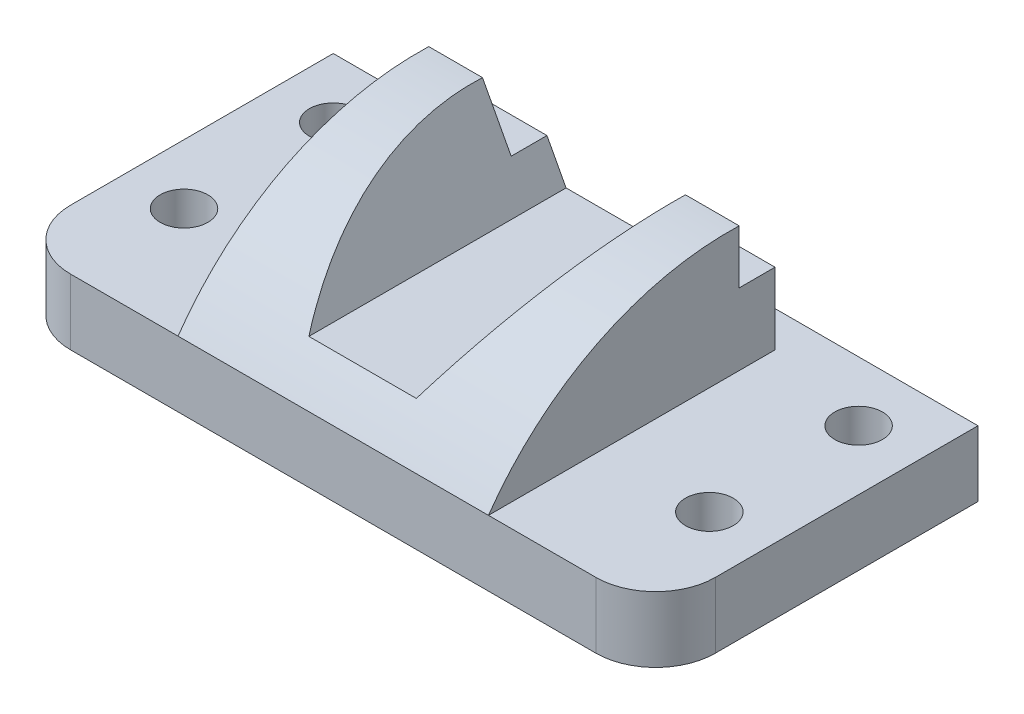
ISO-10303-21;
HEADER;
FILE_DESCRIPTION(('STEP AP214'),'2;1');
FILE_NAME('part.step','',(''),(''),'','','');
FILE_SCHEMA(('AUTOMOTIVE_DESIGN { 1 0 10303 214 1 1 1 1 }'));
ENDSEC;
DATA;
#1=APPLICATION_CONTEXT('core data for automotive mechanical design processes');
#2=APPLICATION_PROTOCOL_DEFINITION('international standard','automotive_design',2000,#1);
#3=PRODUCT_CONTEXT('',#1,'mechanical');
#4=PRODUCT('Part','Part','',(#3));
#5=PRODUCT_RELATED_PRODUCT_CATEGORY('part','',(#4));
#6=PRODUCT_DEFINITION_FORMATION('','',#4);
#7=PRODUCT_DEFINITION_CONTEXT('part definition',#1,'design');
#8=PRODUCT_DEFINITION('design','',#6,#7);
#9=PRODUCT_DEFINITION_SHAPE('','',#8);
#10=(LENGTH_UNIT() NAMED_UNIT(*) SI_UNIT(.MILLI.,.METRE.));
#11=(NAMED_UNIT(*) PLANE_ANGLE_UNIT() SI_UNIT($,.RADIAN.));
#12=(NAMED_UNIT(*) SI_UNIT($,.STERADIAN.) SOLID_ANGLE_UNIT());
#13=UNCERTAINTY_MEASURE_WITH_UNIT(LENGTH_MEASURE(1.E-05),#10,'distance_accuracy_value','');
#14=(GEOMETRIC_REPRESENTATION_CONTEXT(3) GLOBAL_UNCERTAINTY_ASSIGNED_CONTEXT((#13)) GLOBAL_UNIT_ASSIGNED_CONTEXT((#10,
#11,#12)) REPRESENTATION_CONTEXT('',''));
#15=CARTESIAN_POINT('',(0.,0.,0.));
#16=DIRECTION('',(0.,0.,1.));
#17=DIRECTION('',(1.,0.,0.));
#18=AXIS2_PLACEMENT_3D('',#15,#16,#17);
#19=CARTESIAN_POINT('',(-26.,72.,-21.));
#20=DIRECTION('',(0.,0.,1.));
#21=DIRECTION('',(1.,0.,0.));
#22=AXIS2_PLACEMENT_3D('',#19,#20,#21);
#23=PLANE('',#22);
#24=DIRECTION('',(-0.470588235294119,0.88235294117647,0.));
#25=VECTOR('',#24,1.);
#26=CARTESIAN_POINT('',(-35.6020761245675,66.878892733564,-21.));
#27=LINE('',#26,#25);
#28=CARTESIAN_POINT('',(-9.,17.,-21.));
#29=VERTEX_POINT('',#28);
#30=CARTESIAN_POINT('',(-12.2,23.,-21.));
#31=VERTEX_POINT('',#30);
#32=EDGE_CURVE('E178',#29,#31,#27,.T.);
#33=ORIENTED_EDGE('',*,*,#32,.F.);
#34=DIRECTION('',(1.,0.,0.));
#35=VECTOR('',#34,1.);
#36=CARTESIAN_POINT('',(-26.,17.,-21.));
#37=LINE('',#36,#35);
#38=CARTESIAN_POINT('',(9.,17.,-21.));
#39=VERTEX_POINT('',#38);
#40=EDGE_CURVE('E166',#29,#39,#37,.T.);
#41=ORIENTED_EDGE('',*,*,#40,.T.);
#42=DIRECTION('',(0.470588235294118,0.88235294117647,0.));
#43=VECTOR('',#42,1.);
#44=CARTESIAN_POINT('',(24.0865051903114,45.2871972318339,-21.));
#45=LINE('',#44,#43);
#46=CARTESIAN_POINT('',(12.2,23.,-21.));
#47=VERTEX_POINT('',#46);
#48=EDGE_CURVE('E152',#39,#47,#45,.T.);
#49=ORIENTED_EDGE('',*,*,#48,.T.);
#50=DIRECTION('',(1.,0.,0.));
#51=VECTOR('',#50,1.);
#52=CARTESIAN_POINT('',(-35.,23.,-21.));
#53=LINE('',#52,#51);
#54=CARTESIAN_POINT('',(26.,23.,-21.));
#55=VERTEX_POINT('',#54);
#56=EDGE_CURVE('E191',#47,#55,#53,.T.);
#57=ORIENTED_EDGE('',*,*,#56,.T.);
#58=DIRECTION('',(0.,-1.,0.));
#59=VECTOR('',#58,1.);
#60=CARTESIAN_POINT('',(26.,72.,-21.));
#61=LINE('',#60,#59);
#62=CARTESIAN_POINT('',(26.,11.,-21.));
#63=VERTEX_POINT('',#62);
#64=EDGE_CURVE('E211',#55,#63,#61,.T.);
#65=ORIENTED_EDGE('',*,*,#64,.T.);
#66=DIRECTION('',(-1.,0.,0.));
#67=VECTOR('',#66,1.);
#68=CARTESIAN_POINT('',(-26.,11.,-21.));
#69=LINE('',#68,#67);
#70=CARTESIAN_POINT('',(-26.,11.,-21.));
#71=VERTEX_POINT('',#70);
#72=EDGE_CURVE('E202',#63,#71,#69,.T.);
#73=ORIENTED_EDGE('',*,*,#72,.T.);
#74=DIRECTION('',(0.,-1.,0.));
#75=VECTOR('',#74,1.);
#76=CARTESIAN_POINT('',(-26.,72.,-21.));
#77=LINE('',#76,#75);
#78=CARTESIAN_POINT('',(-26.,23.,-21.));
#79=VERTEX_POINT('',#78);
#80=EDGE_CURVE('E65',#79,#71,#77,.T.);
#81=ORIENTED_EDGE('',*,*,#80,.F.);
#82=EDGE_CURVE('E194',#79,#31,#53,.T.);
#83=ORIENTED_EDGE('',*,*,#82,.T.);
#84=EDGE_LOOP('',(#33,#41,#49,#57,#65,#73,#81,#83));
#85=FACE_BOUND('',#84,.T.);
#86=ADVANCED_FACE('F39',(#85),#23,.F.);
#87=CARTESIAN_POINT('',(-35.,23.,-21.));
#88=DIRECTION('',(0.,-1.,0.));
#89=DIRECTION('',(0.,0.,-1.));
#90=AXIS2_PLACEMENT_3D('',#87,#88,#89);
#91=PLANE('',#90);
#92=DIRECTION('',(0.,0.,1.));
#93=VECTOR('',#92,1.);
#94=CARTESIAN_POINT('',(-12.2,23.,-21.));
#95=LINE('',#94,#93);
#96=CARTESIAN_POINT('',(-12.2,23.,-15.));
#97=VERTEX_POINT('',#96);
#98=EDGE_CURVE('E185',#31,#97,#95,.T.);
#99=ORIENTED_EDGE('',*,*,#98,.F.);
#100=ORIENTED_EDGE('',*,*,#82,.F.);
#101=DIRECTION('',(0.,0.,-1.));
#102=VECTOR('',#101,1.);
#103=CARTESIAN_POINT('',(-26.,23.,27.));
#104=LINE('',#103,#102);
#105=CARTESIAN_POINT('',(-26.,23.,-15.));
#106=VERTEX_POINT('',#105);
#107=EDGE_CURVE('E287',#106,#79,#104,.T.);
#108=ORIENTED_EDGE('',*,*,#107,.F.);
#109=DIRECTION('',(1.,0.,0.));
#110=VECTOR('',#109,1.);
#111=CARTESIAN_POINT('',(-35.,23.,-15.));
#112=LINE('',#111,#110);
#113=EDGE_CURVE('E198',#106,#97,#112,.T.);
#114=ORIENTED_EDGE('',*,*,#113,.T.);
#115=EDGE_LOOP('',(#99,#100,#108,#114));
#116=FACE_BOUND('',#115,.T.);
#117=ADVANCED_FACE('F313',(#116),#91,.F.);
#118=CARTESIAN_POINT('',(-35.,23.,-15.));
#119=DIRECTION('',(0.,0.,1.));
#120=DIRECTION('',(1.,0.,0.));
#121=AXIS2_PLACEMENT_3D('',#118,#119,#120);
#122=PLANE('',#121);
#123=DIRECTION('',(-0.470588235294119,0.88235294117647,0.));
#124=VECTOR('',#123,1.);
#125=CARTESIAN_POINT('',(-17.2491349480969,32.4671280276817,-15.));
#126=LINE('',#125,#124);
#127=CARTESIAN_POINT('',(-17.,32.,-15.));
#128=VERTEX_POINT('',#127);
#129=EDGE_CURVE('E162',#97,#128,#126,.T.);
#130=ORIENTED_EDGE('',*,*,#129,.F.);
#131=ORIENTED_EDGE('',*,*,#113,.F.);
#132=DIRECTION('',(0.,-1.,0.));
#133=VECTOR('',#132,1.);
#134=CARTESIAN_POINT('',(-26.,72.,-15.));
#135=LINE('',#134,#133);
#136=CARTESIAN_POINT('',(-26.,32.,-15.));
#137=VERTEX_POINT('',#136);
#138=EDGE_CURVE('E284',#137,#106,#135,.T.);
#139=ORIENTED_EDGE('',*,*,#138,.F.);
#140=DIRECTION('',(1.,0.,0.));
#141=VECTOR('',#140,1.);
#142=CARTESIAN_POINT('',(-35.,32.,-15.));
#143=LINE('',#142,#141);
#144=EDGE_CURVE('E53',#137,#128,#143,.T.);
#145=ORIENTED_EDGE('',*,*,#144,.T.);
#146=EDGE_LOOP('',(#130,#131,#139,#145));
#147=FACE_BOUND('',#146,.T.);
#148=ADVANCED_FACE('F309',(#147),#122,.F.);
#149=CARTESIAN_POINT('',(-35.,-16.9681686592954,-13.2340843296477));
#150=DIRECTION('',(1.,0.,0.));
#151=DIRECTION('',(0.,0.,-1.));
#152=AXIS2_PLACEMENT_3D('',#149,#150,#151);
#153=CYLINDRICAL_SURFACE('',#152,49.);
#154=CARTESIAN_POINT('',(9.11635661829097,-16.9681686592954,-13.2340843296477));
#155=DIRECTION('',(0.88235294117647,0.470588235294119,0.));
#156=DIRECTION('',(0.470588235294119,-0.88235294117647,0.));
#157=AXIS2_PLACEMENT_3D('',#154,#155,#156);
#158=ELLIPSE('',#157,55.5333333333334,49.);
#159=CARTESIAN_POINT('',(-9.,17.,22.0811180332676));
#160=VERTEX_POINT('',#159);
#161=EDGE_CURVE('E11',#128,#160,#158,.T.);
#162=ORIENTED_EDGE('',*,*,#161,.F.);
#163=ORIENTED_EDGE('',*,*,#144,.F.);
#164=CARTESIAN_POINT('',(-26.,-16.9681686592954,-13.2340843296477));
#165=DIRECTION('',(1.,0.,0.));
#166=DIRECTION('',(0.,0.,-1.));
#167=AXIS2_PLACEMENT_3D('',#164,#165,#166);
#168=CIRCLE('',#167,49.);
#169=CARTESIAN_POINT('',(-26.,11.,27.));
#170=VERTEX_POINT('',#169);
#171=EDGE_CURVE('E285',#170,#137,#168,.F.);
#172=ORIENTED_EDGE('',*,*,#171,.F.);
#173=DIRECTION('',(1.,0.,0.));
#174=VECTOR('',#173,1.);
#175=CARTESIAN_POINT('',(-35.,11.,27.));
#176=LINE('',#175,#174);
#177=CARTESIAN_POINT('',(26.,11.,27.));
#178=VERTEX_POINT('',#177);
#179=EDGE_CURVE('E193',#170,#178,#176,.T.);
#180=ORIENTED_EDGE('',*,*,#179,.T.);
#181=CARTESIAN_POINT('',(26.,-16.9681686592954,-13.2340843296477));
#182=DIRECTION('',(-1.,0.,0.));
#183=DIRECTION('',(0.,0.,-1.));
#184=AXIS2_PLACEMENT_3D('',#181,#182,#183);
#185=CIRCLE('',#184,49.);
#186=CARTESIAN_POINT('',(26.,32.,-15.));
#187=VERTEX_POINT('',#186);
#188=EDGE_CURVE('E179',#178,#187,#185,.T.);
#189=ORIENTED_EDGE('',*,*,#188,.T.);
#190=CARTESIAN_POINT('',(17.,32.,-15.));
#191=VERTEX_POINT('',#190);
#192=EDGE_CURVE('E203',#191,#187,#143,.T.);
#193=ORIENTED_EDGE('',*,*,#192,.F.);
#194=CARTESIAN_POINT('',(-9.11635661829093,-16.9681686592954,-13.2340843296477));
#195=DIRECTION('',(0.88235294117647,-0.470588235294118,0.));
#196=DIRECTION('',(0.470588235294118,0.88235294117647,0.));
#197=AXIS2_PLACEMENT_3D('',#194,#195,#196);
#198=ELLIPSE('',#197,55.5333333333334,49.);
#199=CARTESIAN_POINT('',(9.,17.,22.0811180332676));
#200=VERTEX_POINT('',#199);
#201=EDGE_CURVE('E286',#191,#200,#198,.T.);
#202=ORIENTED_EDGE('',*,*,#201,.T.);
#203=DIRECTION('',(1.,0.,0.));
#204=VECTOR('',#203,1.);
#205=CARTESIAN_POINT('',(-35.,17.,22.0811180332676));
#206=LINE('',#205,#204);
#207=EDGE_CURVE('E50',#200,#160,#206,.F.);
#208=ORIENTED_EDGE('',*,*,#207,.T.);
#209=EDGE_LOOP('',(#162,#163,#172,#180,#189,#193,#202,#208));
#210=FACE_BOUND('',#209,.T.);
#211=ADVANCED_FACE('F292',(#210),#153,.T.);
#212=CARTESIAN_POINT('',(26.,72.,-21.));
#213=DIRECTION('',(-1.,0.,0.));
#214=DIRECTION('',(0.,0.,1.));
#215=AXIS2_PLACEMENT_3D('',#212,#213,#214);
#216=PLANE('',#215);
#217=ORIENTED_EDGE('',*,*,#64,.F.);
#218=DIRECTION('',(0.,0.,-1.));
#219=VECTOR('',#218,1.);
#220=CARTESIAN_POINT('',(26.,23.,-21.));
#221=LINE('',#220,#219);
#222=CARTESIAN_POINT('',(26.,23.,-15.));
#223=VERTEX_POINT('',#222);
#224=EDGE_CURVE('E186',#223,#55,#221,.T.);
#225=ORIENTED_EDGE('',*,*,#224,.F.);
#226=DIRECTION('',(0.,-1.,0.));
#227=VECTOR('',#226,1.);
#228=CARTESIAN_POINT('',(26.,23.,-15.));
#229=LINE('',#228,#227);
#230=EDGE_CURVE('E176',#187,#223,#229,.T.);
#231=ORIENTED_EDGE('',*,*,#230,.F.);
#232=ORIENTED_EDGE('',*,*,#188,.F.);
#233=DIRECTION('',(0.,0.,-1.));
#234=VECTOR('',#233,1.);
#235=CARTESIAN_POINT('',(26.,11.,-21.));
#236=LINE('',#235,#234);
#237=EDGE_CURVE('E195',#178,#63,#236,.T.);
#238=ORIENTED_EDGE('',*,*,#237,.T.);
#239=EDGE_LOOP('',(#217,#225,#231,#232,#238));
#240=FACE_BOUND('',#239,.T.);
#241=ADVANCED_FACE('F321',(#240),#216,.F.);
#242=CARTESIAN_POINT('',(-26.,72.,27.));
#243=DIRECTION('',(1.,0.,0.));
#244=DIRECTION('',(0.,0.,-1.));
#245=AXIS2_PLACEMENT_3D('',#242,#243,#244);
#246=PLANE('',#245);
#247=ORIENTED_EDGE('',*,*,#138,.T.);
#248=ORIENTED_EDGE('',*,*,#107,.T.);
#249=ORIENTED_EDGE('',*,*,#80,.T.);
#250=DIRECTION('',(0.,0.,1.));
#251=VECTOR('',#250,1.);
#252=CARTESIAN_POINT('',(-26.,11.,27.));
#253=LINE('',#252,#251);
#254=EDGE_CURVE('E208',#71,#170,#253,.T.);
#255=ORIENTED_EDGE('',*,*,#254,.T.);
#256=ORIENTED_EDGE('',*,*,#171,.T.);
#257=EDGE_LOOP('',(#247,#248,#249,#255,#256));
#258=FACE_BOUND('',#257,.T.);
#259=ADVANCED_FACE('F315',(#258),#246,.F.);
#260=CARTESIAN_POINT('',(-44.,11.,17.));
#261=DIRECTION('',(0.,-1.,0.));
#262=DIRECTION('',(0.,0.,-1.));
#263=AXIS2_PLACEMENT_3D('',#260,#261,#262);
#264=PLANE('',#263);
#265=CARTESIAN_POINT('',(44.,11.,8.00000000000001));
#266=DIRECTION('',(0.,1.,0.));
#267=DIRECTION('',(0.,0.,1.));
#268=AXIS2_PLACEMENT_3D('',#265,#266,#267);
#269=CIRCLE('',#268,4.00000000000001);
#270=CARTESIAN_POINT('',(44.,11.,12.));
#271=VERTEX_POINT('',#270);
#272=EDGE_CURVE('E212',#271,#271,#269,.T.);
#273=ORIENTED_EDGE('',*,*,#272,.F.);
#274=EDGE_LOOP('',(#273));
#275=FACE_BOUND('',#274,.T.);
#276=CARTESIAN_POINT('',(44.,11.,-17.));
#277=DIRECTION('',(0.,1.,0.));
#278=DIRECTION('',(0.,0.,1.));
#279=AXIS2_PLACEMENT_3D('',#276,#277,#278);
#280=CIRCLE('',#279,4.00000000000001);
#281=CARTESIAN_POINT('',(44.,11.,-13.));
#282=VERTEX_POINT('',#281);
#283=EDGE_CURVE('E219',#282,#282,#280,.T.);
#284=ORIENTED_EDGE('',*,*,#283,.F.);
#285=EDGE_LOOP('',(#284));
#286=FACE_BOUND('',#285,.T.);
#287=CARTESIAN_POINT('',(-44.,11.,8.00000000000001));
#288=DIRECTION('',(0.,1.,0.));
#289=DIRECTION('',(0.,0.,1.));
#290=AXIS2_PLACEMENT_3D('',#287,#288,#289);
#291=CIRCLE('',#290,4.00000000000001);
#292=CARTESIAN_POINT('',(-44.,11.,12.));
#293=VERTEX_POINT('',#292);
#294=EDGE_CURVE('E228',#293,#293,#291,.T.);
#295=ORIENTED_EDGE('',*,*,#294,.F.);
#296=EDGE_LOOP('',(#295));
#297=FACE_BOUND('',#296,.T.);
#298=CARTESIAN_POINT('',(-44.,11.,-17.));
#299=DIRECTION('',(0.,1.,0.));
#300=DIRECTION('',(0.,0.,1.));
#301=AXIS2_PLACEMENT_3D('',#298,#299,#300);
#302=CIRCLE('',#301,4.00000000000001);
#303=CARTESIAN_POINT('',(-44.,11.,-13.));
#304=VERTEX_POINT('',#303);
#305=EDGE_CURVE('E234',#304,#304,#302,.T.);
#306=ORIENTED_EDGE('',*,*,#305,.F.);
#307=EDGE_LOOP('',(#306));
#308=FACE_BOUND('',#307,.T.);
#309=ORIENTED_EDGE('',*,*,#254,.F.);
#310=ORIENTED_EDGE('',*,*,#72,.F.);
#311=ORIENTED_EDGE('',*,*,#237,.F.);
#312=DIRECTION('',(1.,0.,0.));
#313=VECTOR('',#312,1.);
#314=CARTESIAN_POINT('',(-43.9999999999999,11.,27.));
#315=LINE('',#314,#313);
#316=CARTESIAN_POINT('',(43.9999999999999,11.,27.));
#317=VERTEX_POINT('',#316);
#318=EDGE_CURVE('E247',#178,#317,#315,.T.);
#319=ORIENTED_EDGE('',*,*,#318,.T.);
#320=CARTESIAN_POINT('',(44.,11.,17.));
#321=DIRECTION('',(0.,1.,0.));
#322=DIRECTION('',(0.,0.,1.));
#323=AXIS2_PLACEMENT_3D('',#320,#321,#322);
#324=CIRCLE('',#323,10.);
#325=CARTESIAN_POINT('',(54.,11.,16.9999999999999));
#326=VERTEX_POINT('',#325);
#327=EDGE_CURVE('E253',#317,#326,#324,.T.);
#328=ORIENTED_EDGE('',*,*,#327,.T.);
#329=DIRECTION('',(0.,0.,-1.));
#330=VECTOR('',#329,1.);
#331=CARTESIAN_POINT('',(54.,11.,16.9999999999999));
#332=LINE('',#331,#330);
#333=CARTESIAN_POINT('',(54.,11.,-27.));
#334=VERTEX_POINT('',#333);
#335=EDGE_CURVE('E236',#326,#334,#332,.T.);
#336=ORIENTED_EDGE('',*,*,#335,.T.);
#337=DIRECTION('',(-1.,0.,0.));
#338=VECTOR('',#337,1.);
#339=CARTESIAN_POINT('',(-54.,11.,-27.));
#340=LINE('',#339,#338);
#341=CARTESIAN_POINT('',(-54.,11.,-27.));
#342=VERTEX_POINT('',#341);
#343=EDGE_CURVE('E243',#334,#342,#340,.T.);
#344=ORIENTED_EDGE('',*,*,#343,.T.);
#345=DIRECTION('',(0.,0.,1.));
#346=VECTOR('',#345,1.);
#347=CARTESIAN_POINT('',(-54.,11.,16.9999999999999));
#348=LINE('',#347,#346);
#349=CARTESIAN_POINT('',(-54.,11.,16.9999999999999));
#350=VERTEX_POINT('',#349);
#351=EDGE_CURVE('E242',#342,#350,#348,.T.);
#352=ORIENTED_EDGE('',*,*,#351,.T.);
#353=CARTESIAN_POINT('',(-44.,11.,17.));
#354=DIRECTION('',(0.,1.,0.));
#355=DIRECTION('',(0.,0.,-1.));
#356=AXIS2_PLACEMENT_3D('',#353,#354,#355);
#357=CIRCLE('',#356,10.);
#358=CARTESIAN_POINT('',(-43.9999999999999,11.,27.));
#359=VERTEX_POINT('',#358);
#360=EDGE_CURVE('E248',#350,#359,#357,.T.);
#361=ORIENTED_EDGE('',*,*,#360,.T.);
#362=EDGE_CURVE('E250',#359,#170,#315,.T.);
#363=ORIENTED_EDGE('',*,*,#362,.T.);
#364=EDGE_LOOP('',(#309,#310,#311,#319,#328,#336,#344,#352,#361,#363));
#365=FACE_BOUND('',#364,.T.);
#366=ADVANCED_FACE('F320',(#275,#286,#297,#308,#365),#264,.F.);
#367=CARTESIAN_POINT('',(-44.,0.,17.));
#368=DIRECTION('',(0.,-1.,0.));
#369=DIRECTION('',(0.,0.,-1.));
#370=AXIS2_PLACEMENT_3D('',#367,#368,#369);
#371=PLANE('',#370);
#372=CARTESIAN_POINT('',(44.,0.,-17.));
#373=DIRECTION('',(0.,1.,0.));
#374=DIRECTION('',(0.,0.,1.));
#375=AXIS2_PLACEMENT_3D('',#372,#373,#374);
#376=CIRCLE('',#375,4.00000000000001);
#377=CARTESIAN_POINT('',(44.,0.,-13.));
#378=VERTEX_POINT('',#377);
#379=EDGE_CURVE('E220',#378,#378,#376,.T.);
#380=ORIENTED_EDGE('',*,*,#379,.T.);
#381=EDGE_LOOP('',(#380));
#382=FACE_BOUND('',#381,.T.);
#383=CARTESIAN_POINT('',(-44.,0.,-17.));
#384=DIRECTION('',(0.,1.,0.));
#385=DIRECTION('',(0.,0.,1.));
#386=AXIS2_PLACEMENT_3D('',#383,#384,#385);
#387=CIRCLE('',#386,4.00000000000001);
#388=CARTESIAN_POINT('',(-44.,0.,-13.));
#389=VERTEX_POINT('',#388);
#390=EDGE_CURVE('E227',#389,#389,#387,.T.);
#391=ORIENTED_EDGE('',*,*,#390,.T.);
#392=EDGE_LOOP('',(#391));
#393=FACE_BOUND('',#392,.T.);
#394=DIRECTION('',(0.,0.,-1.));
#395=VECTOR('',#394,1.);
#396=CARTESIAN_POINT('',(54.,0.,16.9999999999999));
#397=LINE('',#396,#395);
#398=CARTESIAN_POINT('',(54.,0.,16.9999999999999));
#399=VERTEX_POINT('',#398);
#400=CARTESIAN_POINT('',(54.,0.,-27.));
#401=VERTEX_POINT('',#400);
#402=EDGE_CURVE('E231',#399,#401,#397,.T.);
#403=ORIENTED_EDGE('',*,*,#402,.F.);
#404=CARTESIAN_POINT('',(44.,0.,17.));
#405=DIRECTION('',(0.,1.,0.));
#406=DIRECTION('',(0.,0.,1.));
#407=AXIS2_PLACEMENT_3D('',#404,#405,#406);
#408=CIRCLE('',#407,10.);
#409=CARTESIAN_POINT('',(43.9999999999999,0.,27.));
#410=VERTEX_POINT('',#409);
#411=EDGE_CURVE('E245',#410,#399,#408,.T.);
#412=ORIENTED_EDGE('',*,*,#411,.F.);
#413=DIRECTION('',(1.,0.,0.));
#414=VECTOR('',#413,1.);
#415=CARTESIAN_POINT('',(-43.9999999999999,0.,27.));
#416=LINE('',#415,#414);
#417=CARTESIAN_POINT('',(-43.9999999999999,0.,27.));
#418=VERTEX_POINT('',#417);
#419=EDGE_CURVE('E265',#418,#410,#416,.T.);
#420=ORIENTED_EDGE('',*,*,#419,.F.);
#421=CARTESIAN_POINT('',(-44.,0.,17.));
#422=DIRECTION('',(0.,1.,0.));
#423=DIRECTION('',(0.,0.,-1.));
#424=AXIS2_PLACEMENT_3D('',#421,#422,#423);
#425=CIRCLE('',#424,10.);
#426=CARTESIAN_POINT('',(-54.,0.,16.9999999999999));
#427=VERTEX_POINT('',#426);
#428=EDGE_CURVE('E257',#427,#418,#425,.T.);
#429=ORIENTED_EDGE('',*,*,#428,.F.);
#430=DIRECTION('',(0.,0.,1.));
#431=VECTOR('',#430,1.);
#432=CARTESIAN_POINT('',(-54.,0.,16.9999999999999));
#433=LINE('',#432,#431);
#434=CARTESIAN_POINT('',(-54.,0.,-27.));
#435=VERTEX_POINT('',#434);
#436=EDGE_CURVE('E256',#435,#427,#433,.T.);
#437=ORIENTED_EDGE('',*,*,#436,.F.);
#438=DIRECTION('',(-1.,0.,0.));
#439=VECTOR('',#438,1.);
#440=CARTESIAN_POINT('',(-54.,0.,-27.));
#441=LINE('',#440,#439);
#442=EDGE_CURVE('E258',#401,#435,#441,.T.);
#443=ORIENTED_EDGE('',*,*,#442,.F.);
#444=EDGE_LOOP('',(#403,#412,#420,#429,#437,#443));
#445=FACE_BOUND('',#444,.T.);
#446=CARTESIAN_POINT('',(-44.,0.,8.00000000000001));
#447=DIRECTION('',(0.,1.,0.));
#448=DIRECTION('',(0.,0.,1.));
#449=AXIS2_PLACEMENT_3D('',#446,#447,#448);
#450=CIRCLE('',#449,4.00000000000001);
#451=CARTESIAN_POINT('',(-44.,0.,12.));
#452=VERTEX_POINT('',#451);
#453=EDGE_CURVE('E224',#452,#452,#450,.T.);
#454=ORIENTED_EDGE('',*,*,#453,.T.);
#455=EDGE_LOOP('',(#454));
#456=FACE_BOUND('',#455,.T.);
#457=CARTESIAN_POINT('',(44.,0.,8.00000000000001));
#458=DIRECTION('',(0.,1.,0.));
#459=DIRECTION('',(0.,0.,1.));
#460=AXIS2_PLACEMENT_3D('',#457,#458,#459);
#461=CIRCLE('',#460,4.00000000000001);
#462=CARTESIAN_POINT('',(44.,0.,12.));
#463=VERTEX_POINT('',#462);
#464=EDGE_CURVE('E213',#463,#463,#461,.T.);
#465=ORIENTED_EDGE('',*,*,#464,.T.);
#466=EDGE_LOOP('',(#465));
#467=FACE_BOUND('',#466,.T.);
#468=ADVANCED_FACE('F351',(#382,#393,#445,#456,#467),#371,.T.);
#469=CARTESIAN_POINT('',(54.,11.,16.9999999999999));
#470=DIRECTION('',(-1.,0.,0.));
#471=DIRECTION('',(0.,0.,1.));
#472=AXIS2_PLACEMENT_3D('',#469,#470,#471);
#473=PLANE('',#472);
#474=ORIENTED_EDGE('',*,*,#402,.T.);
#475=DIRECTION('',(0.,-1.,0.));
#476=VECTOR('',#475,1.);
#477=CARTESIAN_POINT('',(54.,11.,-27.));
#478=LINE('',#477,#476);
#479=EDGE_CURVE('E276',#334,#401,#478,.T.);
#480=ORIENTED_EDGE('',*,*,#479,.F.);
#481=ORIENTED_EDGE('',*,*,#335,.F.);
#482=DIRECTION('',(0.,-1.,0.));
#483=VECTOR('',#482,1.);
#484=CARTESIAN_POINT('',(54.,11.,16.9999999999999));
#485=LINE('',#484,#483);
#486=EDGE_CURVE('E251',#326,#399,#485,.T.);
#487=ORIENTED_EDGE('',*,*,#486,.T.);
#488=EDGE_LOOP('',(#474,#480,#481,#487));
#489=FACE_BOUND('',#488,.T.);
#490=ADVANCED_FACE('F41',(#489),#473,.F.);
#491=CARTESIAN_POINT('',(-54.,11.,-27.));
#492=DIRECTION('',(0.,0.,1.));
#493=DIRECTION('',(1.,0.,0.));
#494=AXIS2_PLACEMENT_3D('',#491,#492,#493);
#495=PLANE('',#494);
#496=ORIENTED_EDGE('',*,*,#442,.T.);
#497=DIRECTION('',(0.,-1.,0.));
#498=VECTOR('',#497,1.);
#499=CARTESIAN_POINT('',(-54.,11.,-27.));
#500=LINE('',#499,#498);
#501=EDGE_CURVE('E277',#342,#435,#500,.T.);
#502=ORIENTED_EDGE('',*,*,#501,.F.);
#503=ORIENTED_EDGE('',*,*,#343,.F.);
#504=ORIENTED_EDGE('',*,*,#479,.T.);
#505=EDGE_LOOP('',(#496,#502,#503,#504));
#506=FACE_BOUND('',#505,.T.);
#507=ADVANCED_FACE('F337',(#506),#495,.F.);
#508=CARTESIAN_POINT('',(-54.,11.,16.9999999999999));
#509=DIRECTION('',(1.,0.,0.));
#510=DIRECTION('',(0.,0.,-1.));
#511=AXIS2_PLACEMENT_3D('',#508,#509,#510);
#512=PLANE('',#511);
#513=ORIENTED_EDGE('',*,*,#436,.T.);
#514=DIRECTION('',(0.,-1.,0.));
#515=VECTOR('',#514,1.);
#516=CARTESIAN_POINT('',(-54.,11.,16.9999999999999));
#517=LINE('',#516,#515);
#518=EDGE_CURVE('E272',#350,#427,#517,.T.);
#519=ORIENTED_EDGE('',*,*,#518,.F.);
#520=ORIENTED_EDGE('',*,*,#351,.F.);
#521=ORIENTED_EDGE('',*,*,#501,.T.);
#522=EDGE_LOOP('',(#513,#519,#520,#521));
#523=FACE_BOUND('',#522,.T.);
#524=ADVANCED_FACE('F347',(#523),#512,.F.);
#525=CARTESIAN_POINT('',(-44.,11.,17.));
#526=DIRECTION('',(0.,-1.,0.));
#527=DIRECTION('',(0.,0.,-1.));
#528=AXIS2_PLACEMENT_3D('',#525,#526,#527);
#529=CYLINDRICAL_SURFACE('',#528,10.);
#530=ORIENTED_EDGE('',*,*,#428,.T.);
#531=DIRECTION('',(0.,-1.,0.));
#532=VECTOR('',#531,1.);
#533=CARTESIAN_POINT('',(-43.9999999999999,11.,27.));
#534=LINE('',#533,#532);
#535=EDGE_CURVE('E269',#359,#418,#534,.T.);
#536=ORIENTED_EDGE('',*,*,#535,.F.);
#537=ORIENTED_EDGE('',*,*,#360,.F.);
#538=ORIENTED_EDGE('',*,*,#518,.T.);
#539=EDGE_LOOP('',(#530,#536,#537,#538));
#540=FACE_BOUND('',#539,.T.);
#541=ADVANCED_FACE('F348',(#540),#529,.T.);
#542=CARTESIAN_POINT('',(-43.9999999999999,11.,27.));
#543=DIRECTION('',(0.,0.,-1.));
#544=DIRECTION('',(-1.,0.,0.));
#545=AXIS2_PLACEMENT_3D('',#542,#543,#544);
#546=PLANE('',#545);
#547=ORIENTED_EDGE('',*,*,#318,.F.);
#548=ORIENTED_EDGE('',*,*,#179,.F.);
#549=ORIENTED_EDGE('',*,*,#362,.F.);
#550=ORIENTED_EDGE('',*,*,#535,.T.);
#551=ORIENTED_EDGE('',*,*,#419,.T.);
#552=DIRECTION('',(0.,-1.,0.));
#553=VECTOR('',#552,1.);
#554=CARTESIAN_POINT('',(43.9999999999999,11.,27.));
#555=LINE('',#554,#553);
#556=EDGE_CURVE('E270',#317,#410,#555,.T.);
#557=ORIENTED_EDGE('',*,*,#556,.F.);
#558=EDGE_LOOP('',(#547,#548,#549,#550,#551,#557));
#559=FACE_BOUND('',#558,.T.);
#560=ADVANCED_FACE('F330',(#559),#546,.F.);
#561=CARTESIAN_POINT('',(44.,11.,17.));
#562=DIRECTION('',(0.,-1.,0.));
#563=DIRECTION('',(0.,0.,-1.));
#564=AXIS2_PLACEMENT_3D('',#561,#562,#563);
#565=CYLINDRICAL_SURFACE('',#564,10.);
#566=ORIENTED_EDGE('',*,*,#411,.T.);
#567=ORIENTED_EDGE('',*,*,#486,.F.);
#568=ORIENTED_EDGE('',*,*,#327,.F.);
#569=ORIENTED_EDGE('',*,*,#556,.T.);
#570=EDGE_LOOP('',(#566,#567,#568,#569));
#571=FACE_BOUND('',#570,.T.);
#572=ADVANCED_FACE('F331',(#571),#565,.T.);
#573=CARTESIAN_POINT('',(-44.,11.,-17.));
#574=DIRECTION('',(0.,-1.,0.));
#575=DIRECTION('',(0.,0.,-1.));
#576=AXIS2_PLACEMENT_3D('',#573,#574,#575);
#577=CYLINDRICAL_SURFACE('',#576,4.00000000000001);
#578=ORIENTED_EDGE('',*,*,#305,.T.);
#579=EDGE_LOOP('',(#578));
#580=FACE_BOUND('',#579,.T.);
#581=ORIENTED_EDGE('',*,*,#390,.F.);
#582=EDGE_LOOP('',(#581));
#583=FACE_BOUND('',#582,.T.);
#584=ADVANCED_FACE('F485',(#580,#583),#577,.F.);
#585=CARTESIAN_POINT('',(-44.,11.,8.00000000000001));
#586=DIRECTION('',(0.,-1.,0.));
#587=DIRECTION('',(0.,0.,-1.));
#588=AXIS2_PLACEMENT_3D('',#585,#586,#587);
#589=CYLINDRICAL_SURFACE('',#588,4.00000000000001);
#590=ORIENTED_EDGE('',*,*,#294,.T.);
#591=EDGE_LOOP('',(#590));
#592=FACE_BOUND('',#591,.T.);
#593=ORIENTED_EDGE('',*,*,#453,.F.);
#594=EDGE_LOOP('',(#593));
#595=FACE_BOUND('',#594,.T.);
#596=ADVANCED_FACE('F374',(#592,#595),#589,.F.);
#597=CARTESIAN_POINT('',(44.,11.,-17.));
#598=DIRECTION('',(0.,-1.,0.));
#599=DIRECTION('',(0.,0.,-1.));
#600=AXIS2_PLACEMENT_3D('',#597,#598,#599);
#601=CYLINDRICAL_SURFACE('',#600,4.00000000000001);
#602=ORIENTED_EDGE('',*,*,#283,.T.);
#603=EDGE_LOOP('',(#602));
#604=FACE_BOUND('',#603,.T.);
#605=ORIENTED_EDGE('',*,*,#379,.F.);
#606=EDGE_LOOP('',(#605));
#607=FACE_BOUND('',#606,.T.);
#608=ADVANCED_FACE('F364',(#604,#607),#601,.F.);
#609=CARTESIAN_POINT('',(44.,11.,8.00000000000001));
#610=DIRECTION('',(0.,-1.,0.));
#611=DIRECTION('',(0.,0.,-1.));
#612=AXIS2_PLACEMENT_3D('',#609,#610,#611);
#613=CYLINDRICAL_SURFACE('',#612,4.00000000000001);
#614=ORIENTED_EDGE('',*,*,#272,.T.);
#615=EDGE_LOOP('',(#614));
#616=FACE_BOUND('',#615,.T.);
#617=ORIENTED_EDGE('',*,*,#464,.F.);
#618=EDGE_LOOP('',(#617));
#619=FACE_BOUND('',#618,.T.);
#620=ADVANCED_FACE('F362',(#616,#619),#613,.F.);
#621=ORIENTED_EDGE('',*,*,#56,.F.);
#622=DIRECTION('',(0.,0.,1.));
#623=VECTOR('',#622,1.);
#624=CARTESIAN_POINT('',(12.2,23.,-21.));
#625=LINE('',#624,#623);
#626=CARTESIAN_POINT('',(12.2,23.,-15.));
#627=VERTEX_POINT('',#626);
#628=EDGE_CURVE('E157',#47,#627,#625,.T.);
#629=ORIENTED_EDGE('',*,*,#628,.T.);
#630=EDGE_CURVE('E200',#627,#223,#112,.T.);
#631=ORIENTED_EDGE('',*,*,#630,.T.);
#632=ORIENTED_EDGE('',*,*,#224,.T.);
#633=EDGE_LOOP('',(#621,#629,#631,#632));
#634=FACE_BOUND('',#633,.T.);
#635=ADVANCED_FACE('F365',(#634),#91,.F.);
#636=ORIENTED_EDGE('',*,*,#630,.F.);
#637=DIRECTION('',(0.470588235294118,0.88235294117647,0.));
#638=VECTOR('',#637,1.);
#639=CARTESIAN_POINT('',(1.74740484429063,3.40138408304496,-15.));
#640=LINE('',#639,#638);
#641=EDGE_CURVE('E293',#627,#191,#640,.T.);
#642=ORIENTED_EDGE('',*,*,#641,.T.);
#643=ORIENTED_EDGE('',*,*,#192,.T.);
#644=ORIENTED_EDGE('',*,*,#230,.T.);
#645=EDGE_LOOP('',(#636,#642,#643,#644));
#646=FACE_BOUND('',#645,.T.);
#647=ADVANCED_FACE('F296',(#646),#122,.F.);
#648=CARTESIAN_POINT('',(-9.,17.,-34.));
#649=DIRECTION('',(0.,-1.,0.));
#650=DIRECTION('',(0.,0.,-1.));
#651=AXIS2_PLACEMENT_3D('',#648,#649,#650);
#652=PLANE('',#651);
#653=DIRECTION('',(0.,0.,1.));
#654=VECTOR('',#653,1.);
#655=CARTESIAN_POINT('',(-9.,17.,-34.));
#656=LINE('',#655,#654);
#657=EDGE_CURVE('E175',#29,#160,#656,.T.);
#658=ORIENTED_EDGE('',*,*,#657,.T.);
#659=ORIENTED_EDGE('',*,*,#207,.F.);
#660=DIRECTION('',(0.,0.,1.));
#661=VECTOR('',#660,1.);
#662=CARTESIAN_POINT('',(9.,17.,-34.));
#663=LINE('',#662,#661);
#664=EDGE_CURVE('E160',#39,#200,#663,.T.);
#665=ORIENTED_EDGE('',*,*,#664,.F.);
#666=ORIENTED_EDGE('',*,*,#40,.F.);
#667=EDGE_LOOP('',(#658,#659,#665,#666));
#668=FACE_BOUND('',#667,.T.);
#669=ADVANCED_FACE('F169',(#668),#652,.F.);
#670=CARTESIAN_POINT('',(-9.,17.,-34.));
#671=DIRECTION('',(0.88235294117647,0.470588235294119,0.));
#672=DIRECTION('',(-0.470588235294119,0.88235294117647,0.));
#673=AXIS2_PLACEMENT_3D('',#670,#671,#672);
#674=PLANE('',#673);
#675=ORIENTED_EDGE('',*,*,#32,.T.);
#676=ORIENTED_EDGE('',*,*,#98,.T.);
#677=ORIENTED_EDGE('',*,*,#129,.T.);
#678=ORIENTED_EDGE('',*,*,#161,.T.);
#679=ORIENTED_EDGE('',*,*,#657,.F.);
#680=EDGE_LOOP('',(#675,#676,#677,#678,#679));
#681=FACE_BOUND('',#680,.T.);
#682=ADVANCED_FACE('F308',(#681),#674,.T.);
#683=CARTESIAN_POINT('',(9.,17.,-34.));
#684=DIRECTION('',(0.88235294117647,-0.470588235294118,0.));
#685=DIRECTION('',(0.470588235294118,0.88235294117647,0.));
#686=AXIS2_PLACEMENT_3D('',#683,#684,#685);
#687=PLANE('',#686);
#688=ORIENTED_EDGE('',*,*,#664,.T.);
#689=ORIENTED_EDGE('',*,*,#201,.F.);
#690=ORIENTED_EDGE('',*,*,#641,.F.);
#691=ORIENTED_EDGE('',*,*,#628,.F.);
#692=ORIENTED_EDGE('',*,*,#48,.F.);
#693=EDGE_LOOP('',(#688,#689,#690,#691,#692));
#694=FACE_BOUND('',#693,.T.);
#695=ADVANCED_FACE('F156',(#694),#687,.F.);
#696=CLOSED_SHELL('',(#86,#117,#148,#211,#241,#259,#366,#468,#490,#507,#524,#541,#560,#572,#584,
#596,#608,#620,#635,#647,#669,#682,#695));
#697=MANIFOLD_SOLID_BREP('B2',#696);
#698=ADVANCED_BREP_SHAPE_REPRESENTATION('',(#18,#697),#14);
#699=SHAPE_DEFINITION_REPRESENTATION(#9,#698);
ENDSEC;
END-ISO-10303-21;
